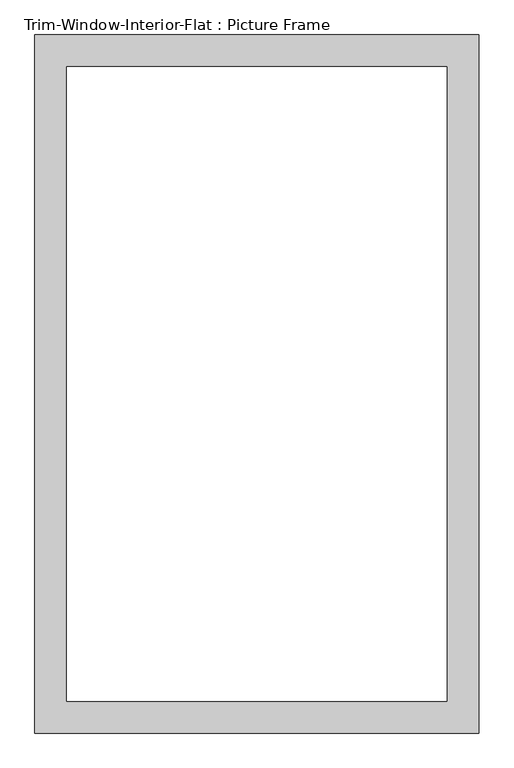
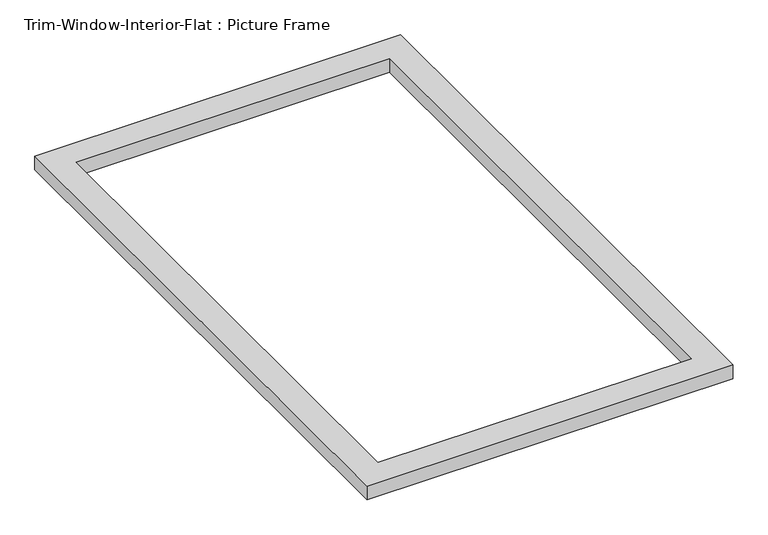
"""IFC4 building model written with IfcOpenShell, lengths in millimetres: proxy geometry, Trim-Window-Interior-Flat : Picture Frame."""

from ifc_helpers import new_model, si_unit, origin, origin_with_axes, place, context, project, spatial, polyline, outline, extrude, source, transform, mapped, element, save


def trim_window_interior_flat_picture_frame_d3d93820(model_context):
    return source(origin(), model_context, "Body", "SweptSolid", [
        extrude(outline(polyline([(400.05, 44.45), (400.05, -1212.85), (-400.05, -1212.85), (-400.05, 44.45), (400.05, 44.45)]), holes=[polyline([(342.9, -12.7), (-342.9, -12.7), (-342.9, -1155.7), (342.9, -1155.7), (342.9, -12.7)])]), origin_with_axes(), (0.0, 0.0, 1.0), 31.75),
    ])


if __name__ == "__main__":
    model = new_model("IFC4")
    model_context = context("Model", 3, world=origin())
    ifc_project = project(units=[si_unit("LENGTHUNIT", "METRE", prefix="MILLI")], contexts=[model_context])
    site = spatial("IfcSite", under=ifc_project)
    building = spatial("IfcBuilding", under=site)
    placement = place(None, origin())
    trim_window_interior_flat_picture_frame_shape = trim_window_interior_flat_picture_frame_d3d93820(model_context)
    element("IfcBuildingElementProxy", 1, Name="Trim-Window-Interior-Flat : Picture Frame", ObjectType="Trim-Window-Interior-Flat : Picture Frame", at=placement, inside=building, context=model_context, shape_type="MappedRepresentation", body=[
        mapped(trim_window_interior_flat_picture_frame_shape, transform((0.0, 0.0, 0.0), x_axis=(1.0, 0.0, 0.0), y_axis=(0.0, 1.0, 0.0), z_axis=(0.0, 0.0, 1.0))),
    ])
    save(model, "model.ifc")

# Revit data of these elements
# Type "Trim-Window-Interior-Flat : Picture Frame"
#   Trim Thickness_Picture Frame = 0' - 1 1/4"
#   Trim Width = 0' - 2 1/4"
#   Trim Thickness_with Sill = 0' - 0 3/4"
#   Sill Thickness = 0' - 1 1/4"
#   Opening Width [instance default] = 2' - 0"
#   Opening Height [instance default] = 3' - 0"
#   Default Elevation = 4' - 0"
#   Sill = no
#   Picture Frame = yes
#   Trim Material [instance default] = none
# Element 1 (IfcBuildingElementProxy, "Trim-Window-Interior-Flat : Picture Frame")
#   Opening Width = 2' - 4"
#   Opening Height = 3' - 10"
#   Trim Material = Wood - Stained
#   Materials on its faces: "Wood - Stained"
# Materials
#   "Wood - Stained": class "Wood", colour RGB 224 178 126, transparency 0, Cost = 0
